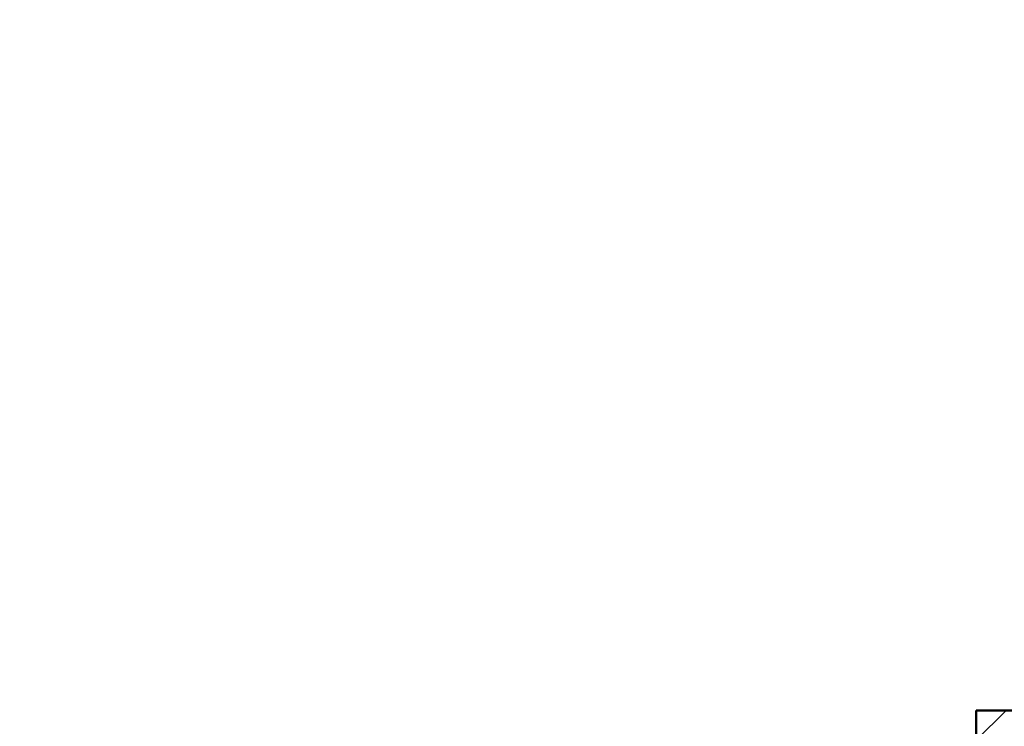
# Model space of a CAD drawing. Units: inches. Extents: x 1901 to 2863, y 888 to 2433.
# Tile 72 of 91: x 2529 to 2608, y 2009 to 2066. Entities that reach past the tile are written whole.
import ezdxf

# ---------------------------------------------------------------- set-up
doc = ezdxf.new("R2010")
doc.units = ezdxf.units.IN
doc.layers.add('A-WALL', color=7, linetype='Continuous', lineweight=50)
doc.layers.add('A-WALL-PATT', color=8, linetype='Continuous', lineweight=13)

msp = doc.modelspace()

# ---------------------------------------------------------------- hatches: boundary and pattern name
at = {"layer": 'A-WALL-PATT'}
h = msp.add_hatch(dxfattribs=at)
h.set_pattern_fill('ANSI32', color=256)
h.paths.add_polyline_path([(2192.501, 2274.134), (2141.264, 2274.134), (2141.264, 2269.634), (2192.501, 2269.634)])
h.paths.add_polyline_path([(2259.926, 2274.134), (2216.501, 2274.134), (2216.501, 2269.634), (2255.426, 2269.634), (2255.426, 2214.634), (2250.809, 2214.634), (2250.809, 2210.134), (2259.926, 2210.134), (2259.926, 2215.134), (2271.756, 2215.134), (2271.756, 2217.384), (2271.756, 2219.634), (2259.926, 2219.634)])
h.paths.add_polyline_path([(2171.426, 2269.634), (2166.926, 2269.634), (2166.926, 2219.634), (2121.238, 2219.634), (2121.238, 2215.134), (2166.926, 2215.134), (2166.926, 2083.134), (2161.807, 2083.134), (2161.807, 2078.634), (2171.426, 2078.634), (2176.996, 2078.634), (2176.996, 2080.884), (2176.996, 2083.134), (2171.426, 2083.134), (2171.426, 2210.134), (2230.912, 2210.134), (2230.912, 2212.384), (2230.912, 2214.634), (2171.426, 2214.634)])
h.paths.add_polyline_path([(2117.264, 2274.134), (2089.426, 2274.134), (2089.426, 2219.634), (2081.136, 2219.634), (2081.136, 2215.134), (2089.426, 2215.134), (2098.004, 2215.134), (2098.004, 2217.384), (2098.004, 2219.634), (2093.926, 2219.634), (2093.926, 2269.634), (2117.264, 2269.634), (2117.264, 2271.884)])
h.paths.add_polyline_path([(2343.426, 2219.634), (2329.295, 2219.634), (2329.295, 2215.134), (2338.926, 2215.134), (2338.926, 2184.739), (2343.426, 2184.739)])
h.paths.add_polyline_path([(2338.926, 2083.134), (2329.295, 2083.134), (2208.966, 2083.134), (2208.966, 2078.634), (2338.926, 2078.634)])
h.paths.add_polyline_path([(2343.426, 2136.739), (2338.926, 2136.739), (2338.926, 1872.634), (2343.426, 1872.634)])
h.paths.add_polyline_path([(2343.426, 1863.634), (2397.68, 1863.634), (2397.68, 1821.634), (2384.138, 1821.634), (2384.138, 1812.634), (2418.33, 1812.634), (2418.33, 1817.134), (2418.33, 1821.634), (2406.68, 1821.634), (2406.68, 1863.634), (2459.499, 1863.634), (2459.499, 1821.634), (2447.138, 1821.634), (2447.138, 1812.634), (2459.499, 1812.634), (2468.499, 1812.634), (2468.499, 1872.634), (2394.426, 1872.634), (2334.426, 1872.634), (2334.426, 1812.634), (2343.426, 1812.634), (2353.251, 1812.634), (2353.251, 1821.634), (2343.426, 1821.634)])
h.paths.add_polyline_path([(2510.014, 1872.634), (2468.499, 1872.634), (2468.499, 1868.134), (2510.014, 1868.134)])
h.paths.add_polyline_path([(2514.009, 1817.134), (2468.499, 1817.134), (2468.499, 1812.634), (2482.114, 1812.634), (2482.114, 1800.606), (2486.614, 1800.606), (2486.614, 1812.634), (2514.009, 1812.634)])
h.paths.add_polyline_path([(2299.247, 1814.884), (2299.247, 1817.134), (2295.926, 1817.134), (2295.926, 1854.169), (2293.676, 1854.169), (2291.426, 1854.169), (2291.426, 1817.134), (2266.109, 1817.134), (2266.109, 1812.634), (2299.247, 1812.634)])
h.paths.add_polyline_path([(2218.109, 1817.134), (2206.46, 1817.134), (2171.426, 1817.134), (2171.426, 1949.134), (2190.1, 1949.134), (2190.1, 1953.634), (2163.468, 1953.634), (2163.468, 1949.134), (2166.926, 1949.134), (2166.926, 1817.134), (2114.297, 1817.134), (2114.297, 1812.634), (2218.109, 1812.634)])
h.paths.add_polyline_path([(2029.426, 1970.922), (2024.926, 1970.922), (2024.926, 1912.717), (2029.426, 1912.717)])
h.paths.add_polyline_path([(2132.297, 1953.634), (2113.926, 1953.634), (2113.926, 1975.888), (2111.676, 1975.888), (2109.426, 1975.888), (2109.426, 1953.634), (2029.426, 1953.634), (2029.426, 1949.134), (2132.297, 1949.134)])
h.paths.add_polyline_path([(2029.426, 1853.606), (2029.31, 1853.606), (2029.31, 1853.606), (2029.426, 1853.606), (2029.426, 1864.717), (2024.926, 1864.717), (2024.926, 1812.634), (2066.297, 1812.634), (2066.297, 1814.884), (2066.297, 1817.134), (2029.426, 1817.134)])
h.paths.add_polyline_path([(2122.926, 2010.088), (2120.676, 2010.088), (2118.426, 2010.088), (2118.426, 2006.134), (2029.426, 2006.134), (2029.426, 2001.634), (2109.426, 2001.634), (2109.426, 1998.041), (2113.926, 1998.041), (2113.926, 2001.634), (2122.926, 2001.634)])
h.paths.add_polyline_path([(2029.426, 2031.376), (2024.926, 2031.376), (2024.926, 1994.922), (2027.176, 1994.922), (2029.426, 1994.922)])
h.paths.add_polyline_path([(2029.426, 2136.739), (2024.926, 2136.739), (2024.926, 2067.376), (2027.176, 2067.376), (2029.426, 2067.376)])
h.paths.add_polyline_path([(2125.618, 2083.134), (2029.426, 2083.134), (2029.426, 2078.634), (2118.426, 2078.634), (2118.426, 2030.715), (2122.926, 2030.715), (2122.926, 2078.634), (2125.618, 2078.634)])
h.paths.add_polyline_path([(2029.426, 2215.134), (2040.468, 2215.134), (2040.468, 2217.384), (2040.468, 2219.634), (2024.926, 2219.634), (2024.926, 2184.739), (2029.426, 2184.739), (2029.426, 2187.778)])
h.paths.add_polyline_path([(2686.426, 2274.134), (2659.284, 2274.134), (2659.284, 2269.634), (2681.926, 2269.634), (2681.926, 2219.634), (2676.816, 2219.634), (2676.816, 2215.134), (2681.926, 2215.134), (2697.011, 2215.134), (2697.011, 2217.384), (2697.011, 2219.634), (2686.426, 2219.634)])
h.paths.add_polyline_path([(2609.926, 2269.634), (2635.284, 2269.634), (2635.284, 2274.134), (2571.431, 2274.134), (2571.431, 2269.634), (2605.426, 2269.634), (2605.426, 2214.634), (2549.098, 2214.634), (2549.098, 2210.134), (2605.426, 2210.134), (2605.426, 2083.134), (2601.014, 2083.134), (2601.014, 2080.884), (2601.014, 2078.634), (2609.926, 2078.634), (2616.162, 2078.634), (2616.162, 2080.884), (2616.162, 2083.134), (2609.926, 2083.134), (2609.926, 2215.134), (2651.465, 2215.134), (2651.465, 2217.384), (2651.465, 2219.634), (2609.926, 2219.634)])
h.paths.add_polyline_path([(2521.426, 2269.634), (2547.431, 2269.634), (2547.431, 2271.884), (2547.431, 2274.134), (2516.926, 2274.134), (2516.926, 2219.634), (2506.41, 2219.634), (2506.41, 2215.134), (2516.926, 2215.134), (2516.926, 2210.134), (2525.402, 2210.134), (2525.402, 2212.384), (2525.402, 2214.634), (2521.426, 2214.634)])
h.paths.add_polyline_path([(2456.011, 2219.634), (2439.426, 2219.634), (2439.426, 2187.888), (2443.926, 2187.888), (2443.926, 2215.134), (2456.011, 2215.134)])
h.paths.add_polyline_path([(2752.926, 2219.634), (2739.485, 2219.634), (2739.485, 2215.134), (2748.426, 2215.134), (2748.426, 2187.888), (2752.926, 2187.888)])
h.paths.add_polyline_path([(2752.926, 2139.888), (2748.426, 2139.888), (2748.426, 2083.134), (2648.416, 2083.134), (2648.416, 2078.634), (2654.926, 2078.634), (2654.926, 2039.437), (2659.426, 2039.437), (2659.426, 2078.634), (2748.426, 2078.634), (2748.426, 2063.429), (2752.926, 2063.429)])
h.paths.add_polyline_path([(2752.926, 2010.634), (2659.426, 2010.634), (2659.426, 2015.652), (2654.926, 2015.652), (2654.926, 2010.634), (2605.426, 2010.634), (2605.426, 1920.967), (2609.926, 1920.967), (2609.926, 2006.134), (2748.426, 2006.134), (2748.426, 1982.466), (2752.926, 1982.466)])
h.paths.add_polyline_path([(2752.926, 2027.429), (2748.426, 2027.429), (2748.426, 2010.634), (2752.926, 2010.634)])
h.paths.add_polyline_path([(2748.426, 1886.134), (2609.926, 1886.134), (2609.926, 1889.719), (2605.426, 1889.719), (2605.426, 1861.262), (2609.926, 1861.262), (2609.926, 1881.634), (2748.426, 1881.634)])
h.paths.add_polyline_path([(2456.855, 2228.831), (2498.401, 2228.831), (2498.401, 2247.488), (2456.855, 2247.488)], flags=9)
h.paths.add_polyline_path([(2038.602, 2237.418), (2080.174, 2237.418), (2080.174, 2256.075), (2038.602, 2256.075)], flags=9)
h.paths.add_polyline_path([(2292.009, 1062.394), (2539.932, 1062.394), (2539.932, 1099.487), (2292.009, 1099.487)], flags=9)
h.paths.add_polyline_path([(2424.91, 1832.253), (2448.513, 1832.253), (2448.513, 1846.678), (2424.91, 1846.678)], flags=25)
h.paths.add_polyline_path([(2359.076, 1832.253), (2382.678, 1832.253), (2382.678, 1846.678), (2359.076, 1846.678)], flags=25)
h.paths.add_polyline_path([(2352.899, 1684.802), (2367.543, 1684.802), (2367.543, 1697.167), (2352.899, 1697.167)], flags=9)
h.paths.add_polyline_path([(2079.288, 1755.826), (2169.024, 1755.826), (2169.024, 1774.372), (2079.288, 1774.372)], flags=9)
h.paths.add_polyline_path([(2404.09, 1373.857), (2404.09, 1463.593), (2385.544, 1463.593), (2385.544, 1373.857)], flags=9)
h.paths.add_polyline_path([(2268.091, 2236.371), (2309.636, 2236.371), (2309.636, 2255.028), (2268.091, 2255.028)], flags=9)
h.paths.add_polyline_path([(2575.96, 1700.951), (2665.696, 1700.951), (2665.696, 1719.498), (2575.96, 1719.498)], flags=9)
h.paths.add_polyline_path([(2302.962, 1878.474), (2329.524, 1878.474), (2329.524, 1888.777), (2302.962, 1888.777)], flags=9)
h.paths.add_polyline_path([(2097.415, 2240.576), (2126.573, 2240.576), (2126.573, 2259.233), (2097.415, 2259.233)], flags=9)
h.paths.add_polyline_path([(2208.725, 2246.124), (2237.882, 2246.124), (2237.882, 2264.781), (2208.725, 2264.781)], flags=9)
h.paths.add_polyline_path([(2038.147, 1925.958), (2076.987, 1925.958), (2076.987, 1944.615), (2038.147, 1944.615)], flags=9)
h.paths.add_polyline_path([(2239.144, 1926.672), (2288.465, 1926.672), (2288.465, 1945.329), (2239.144, 1945.329)], flags=9)
h.paths.add_polyline_path([(2175.429, 2007.33), (2212.356, 2007.33), (2212.356, 2025.987), (2175.429, 2025.987)], flags=9)
h.paths.add_polyline_path([(2225.034, 2091.794), (2263.875, 2091.794), (2263.875, 2110.451), (2225.034, 2110.451)], flags=9)
h.paths.add_polyline_path([(2035.398, 2098.478), (2074.238, 2098.478), (2074.238, 2117.135), (2035.398, 2117.135)], flags=9)
h.paths.add_polyline_path([(2050.102, 2029.209), (2083.26, 2029.209), (2083.26, 2047.866), (2050.102, 2047.866)], flags=9)
h.paths.add_polyline_path([(2069.677, 1956.719), (2098.835, 1956.719), (2098.835, 1975.376), (2069.677, 1975.376)], flags=25)
h.paths.add_polyline_path([(2328.62, 1753.336), (2361.663, 1753.336), (2361.663, 1771.993), (2328.62, 1771.993)], flags=9)
h.paths.add_polyline_path([(2395.162, 2060.888), (2395.162, 2140.654), (2378.676, 2140.654), (2378.676, 2060.888)], flags=9)
h.paths.add_polyline_path([(2463.728, 2059.02), (2492.886, 2059.02), (2492.886, 2077.677), (2463.728, 2077.677)], flags=9)
h.paths.add_polyline_path([(2458.027, 2181.536), (2496.868, 2181.536), (2496.868, 2200.194), (2458.027, 2200.194)], flags=9)
h.paths.add_polyline_path([(2527.577, 2243.074), (2556.735, 2243.074), (2556.735, 2261.731), (2527.577, 2261.731)], flags=9)
h.paths.add_polyline_path([(2694.461, 2232.767), (2736.033, 2232.767), (2736.033, 2251.425), (2694.461, 2251.425)], flags=9)
h.paths.add_polyline_path([(2637.821, 2249.225), (2666.979, 2249.225), (2666.979, 2267.882), (2637.821, 2267.882)], flags=9)
h.paths.add_polyline_path([(2623.687, 2183.541), (2662.528, 2183.541), (2662.528, 2202.199), (2623.687, 2202.199)], flags=9)
h.paths.add_polyline_path([(2691.965, 2021.5), (2725.124, 2021.5), (2725.124, 2040.157), (2691.965, 2040.157)], flags=9)
h.paths.add_polyline_path([(2621.043, 1975.912), (2662.335, 1975.912), (2662.335, 1994.569), (2621.043, 1994.569)], flags=25)
h.paths.add_polyline_path([(2479.032, 1927.62), (2519.844, 1927.62), (2519.844, 1946.277), (2479.032, 1946.277)], flags=9)
h.paths.add_polyline_path([(2670.941, 1849.076), (2716.005, 1849.076), (2716.005, 1867.734), (2670.941, 1867.734)], flags=9)
h.paths.add_polyline_path([(2523.613, 1782.956), (2550.175, 1782.956), (2550.175, 1793.26), (2523.613, 1793.26)], flags=9)
h.paths.add_polyline_path([(2450.841, 1207.331), (2492.386, 1207.331), (2492.386, 1225.989), (2450.841, 1225.989)], flags=9)
h.paths.add_polyline_path([(2527.751, 1203.841), (2556.908, 1203.841), (2556.908, 1222.499), (2527.751, 1222.499)], flags=9)
h.paths.add_polyline_path([(2639.111, 1207.2), (2668.268, 1207.2), (2668.268, 1225.857), (2639.111, 1225.857)], flags=9)
h.paths.add_polyline_path([(2692.594, 1218.965), (2734.167, 1218.965), (2734.167, 1237.623), (2692.594, 1237.623)], flags=9)
h.paths.add_polyline_path([(2669.266, 1366.329), (2708.106, 1366.329), (2708.106, 1384.987), (2669.266, 1384.987)], flags=9)
h.paths.add_polyline_path([(2463.313, 1358.031), (2502.153, 1358.031), (2502.153, 1376.688), (2463.313, 1376.688)], flags=9)
h.paths.add_polyline_path([(2494.725, 1449.963), (2531.652, 1449.963), (2531.652, 1468.62), (2494.725, 1468.62)], flags=9)
h.paths.add_polyline_path([(2675.565, 1422.157), (2708.724, 1422.157), (2708.724, 1440.815), (2675.565, 1440.815)], flags=9)
h.paths.add_polyline_path([(2685.634, 1493.891), (2714.792, 1493.891), (2714.792, 1512.548), (2685.634, 1512.548)], flags=9)
h.paths.add_polyline_path([(2686.805, 1529.913), (2725.645, 1529.913), (2725.645, 1548.57), (2686.805, 1548.57)], flags=9)
h.paths.add_polyline_path([(2503.651, 1537.991), (2552.972, 1537.991), (2552.972, 1556.648), (2503.651, 1556.648)], flags=9)
h.paths.add_polyline_path([(2291.713, 1643.504), (2318.275, 1643.504), (2318.275, 1653.807), (2291.713, 1653.807)], flags=9)
h.paths.add_polyline_path([(2450.626, 1610.52), (2477.189, 1610.52), (2477.189, 1620.824), (2450.626, 1620.824)], flags=9)
h.paths.add_polyline_path([(2359.985, 1551.814), (2422.253, 1551.814), (2422.253, 1562.117), (2359.985, 1562.117)], flags=9)
h.paths.add_polyline_path([(2280.106, 1249.006), (2321.651, 1249.006), (2321.651, 1267.663), (2280.106, 1267.663)], flags=9)
h.paths.add_polyline_path([(2164.057, 1274.232), (2193.215, 1274.232), (2193.215, 1292.889), (2164.057, 1292.889)], flags=9)
h.paths.add_polyline_path([(2118.21, 1277.694), (2151.252, 1277.694), (2151.252, 1296.351), (2118.21, 1296.351)], flags=9)
h.paths.add_polyline_path([(2031.946, 1268.529), (2073.519, 1268.529), (2073.519, 1287.187), (2031.946, 1287.187)], flags=9)
h.paths.add_polyline_path([(2050.199, 1409.079), (2089.04, 1409.079), (2089.04, 1427.736), (2050.199, 1427.736)], flags=9)
h.paths.add_polyline_path([(2243.743, 1421.032), (2282.584, 1421.032), (2282.584, 1439.689), (2243.743, 1439.689)], flags=9)
h.paths.add_polyline_path([(2190.746, 1509.769), (2231.558, 1509.769), (2231.558, 1528.426), (2190.746, 1528.426)], flags=9)
h.paths.add_polyline_path([(2058.392, 1475.415), (2091.55, 1475.415), (2091.55, 1494.073), (2058.392, 1494.073)], flags=9)
h.paths.add_polyline_path([(2062.447, 1553.09), (2091.605, 1553.09), (2091.605, 1571.747), (2062.447, 1571.747)], flags=9)
h.paths.add_polyline_path([(2219.524, 1590.365), (2266.147, 1590.365), (2266.147, 1609.022), (2219.524, 1609.022)], flags=9)
h.paths.add_polyline_path([(2041.072, 1584.188), (2079.912, 1584.188), (2079.912, 1602.845), (2041.072, 1602.845)], flags=9)

# ---------------------------------------------------------------- linework, layer by layer
at = {"layer": 'A-WALL'}
for p, q in [((2605.426, 2010.634), (2605.426, 1920.967)), ((2654.926, 2010.634), (2605.426, 2010.634))]:
    msp.add_line(p, q, dxfattribs=at)

doc.saveas('drawing.dxf')
